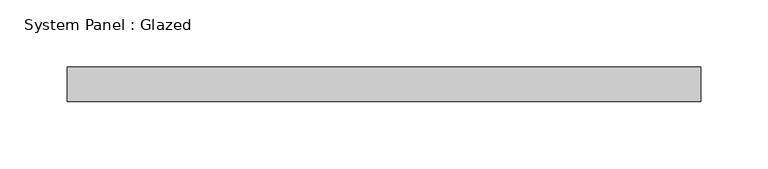
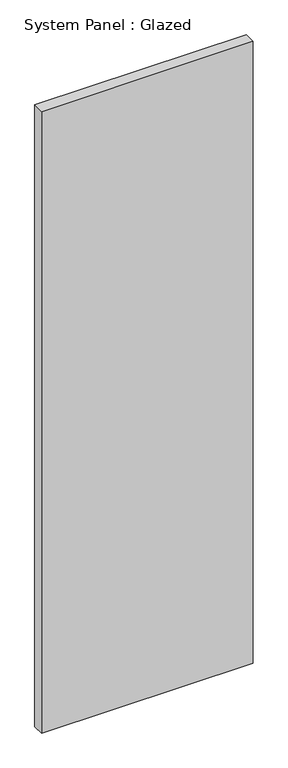
"""IFC4 building model written with IfcOpenShell, lengths in millimetres: plate geometry, System Panel : Glazed."""

from ifc_helpers import new_model, si_unit, origin, origin_with_axes, place, context, project, spatial, polyline, outline, extrude, source, transform, mapped, element, save


def system_panel_glazed_d4004c69(model_context):
    return source(origin(), model_context, "Body", "SweptSolid", [
        extrude(outline(polyline([(234.95, 19.05), (-234.95, 19.05), (-234.95, 44.45), (234.95, 44.45), (234.95, 19.05)])), origin_with_axes(), (0.0, 0.0, 1.0), 1459.1267095),
    ])


if __name__ == "__main__":
    model = new_model("IFC4")
    model_context = context("Model", 3, world=origin())
    ifc_project = project(units=[si_unit("LENGTHUNIT", "METRE", prefix="MILLI")], contexts=[model_context])
    site = spatial("IfcSite", under=ifc_project)
    building = spatial("IfcBuilding", under=site)
    placement = place(None, origin())
    system_panel_glazed_shape = system_panel_glazed_d4004c69(model_context)
    element("IfcPlate", 1, ObjectType="System Panel : Glazed", at=placement, inside=building, context=model_context, shape_type="MappedRepresentation", body=[
        mapped(system_panel_glazed_shape, transform((0.0, 0.0, 0.0), x_axis=(1.0, 0.0, 0.0), y_axis=(0.0, 1.0, 0.0), z_axis=(0.0, 0.0, 1.0))),
    ])
    save(model, "model.ifc")

# Revit data of these elements
# Type "System Panel : Glazed"
#   Construction Type Id = "GSP4R"
#   Analytic Construction = "1/8 in Pilkington single glazing"
#   Visual Light Transmittance = 0.9
#   Solar Heat Gain Coefficient = 0.86
#   Heat Transfer Coefficient (U) = 1.18115 BTU/(h·ft²·°F)
#   Define Thermal Properties by = 1
# Element 1 (IfcPlate, "System Panel : Glazed")
#   Materials on its faces: "Glass"
# Materials
#   "Glass": class "Glass", colour RGB 0 128 192, transparency 0.75, Description = "Soda Lime Glass", Cost = 0
